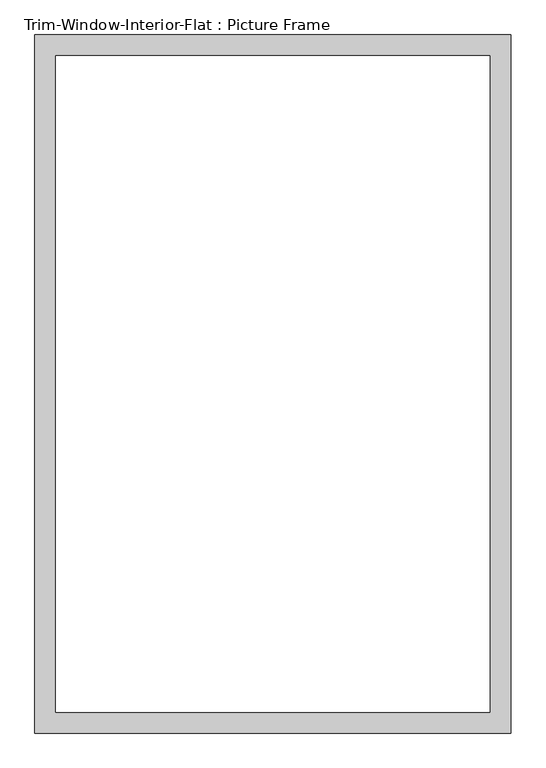
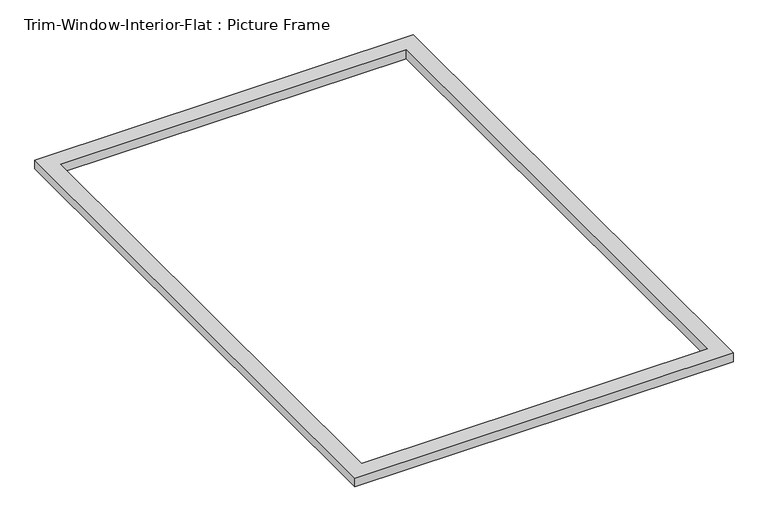
"""IFC4 building model written with IfcOpenShell, lengths in millimetres: proxy geometry, Trim-Window-Interior-Flat : Picture Frame."""

from ifc_helpers import new_model, si_unit, origin, origin_with_axes, place, context, project, spatial, polyline, outline, extrude, source, transform, mapped, element, save


def trim_window_interior_flat_picture_frame_936b8d2a(model_context):
    return source(origin(), model_context, "Body", "SweptSolid", [
        extrude(outline(polyline([(654.05, 44.45), (654.05, -1873.25), (-654.05, -1873.25), (-654.05, 44.45), (654.05, 44.45)]), holes=[polyline([(596.9, -12.7), (-596.9, -12.7), (-596.9, -1816.1), (596.9, -1816.1), (596.9, -12.7)])]), origin_with_axes(), (0.0, 0.0, 1.0), 31.75),
    ])


if __name__ == "__main__":
    model = new_model("IFC4")
    model_context = context("Model", 3, world=origin())
    ifc_project = project(units=[si_unit("LENGTHUNIT", "METRE", prefix="MILLI")], contexts=[model_context])
    site = spatial("IfcSite", under=ifc_project)
    building = spatial("IfcBuilding", under=site)
    placement = place(None, origin())
    trim_window_interior_flat_picture_frame_shape = trim_window_interior_flat_picture_frame_936b8d2a(model_context)
    element("IfcBuildingElementProxy", 1, Name="Trim-Window-Interior-Flat : Picture Frame", ObjectType="Trim-Window-Interior-Flat : Picture Frame", at=placement, inside=building, context=model_context, shape_type="MappedRepresentation", body=[
        mapped(trim_window_interior_flat_picture_frame_shape, transform((0.0, 0.0, 0.0), x_axis=(1.0, 0.0, 0.0), y_axis=(0.0, 1.0, 0.0), z_axis=(0.0, 0.0, 1.0))),
    ])
    save(model, "model.ifc")

# Revit data of these elements
# Type "Trim-Window-Interior-Flat : Picture Frame"
#   Trim Thickness_Picture Frame = 0' - 1 1/4"
#   Trim Width = 0' - 2 1/4"
#   Trim Thickness_with Sill = 0' - 0 3/4"
#   Sill Thickness = 0' - 1 1/4"
#   Opening Width [instance default] = 2' - 0"
#   Opening Height [instance default] = 3' - 0"
#   Default Elevation = 4' - 0"
#   Sill = no
#   Picture Frame = yes
#   Trim Material [instance default] = none
# Element 1 (IfcBuildingElementProxy, "Trim-Window-Interior-Flat : Picture Frame")
#   Opening Width = 4' - 0"
#   Opening Height = 6' - 0"
#   Trim Material = Wood - Stained
#   Materials on its faces: "Wood - Stained"
# Materials
#   "Wood - Stained": class "Wood", colour RGB 224 178 126, transparency 0, Cost = 0
